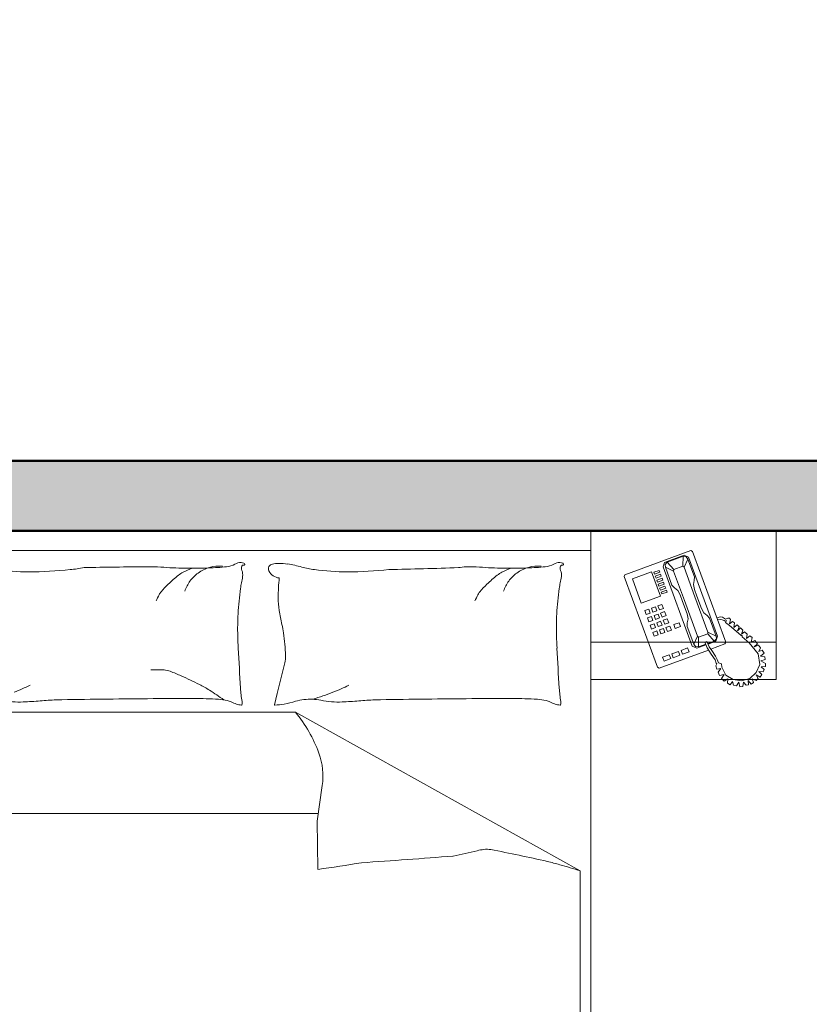
# Model space of a CAD drawing. Units: inches. Extents: x -7 to 1228, y -146 to 1091.
# Tile 32 of 88: x 680 to 747, y 446 to 531. Entities that reach past the tile are written whole.
import ezdxf

# ---------------------------------------------------------------- set-up
doc = ezdxf.new("R2010")
doc.units = ezdxf.units.IN
for name, color, linetype, lineweight in [('A-FURN', 8, 'Continuous', 18), ('A-WALL', 7, 'Continuous', 50), ('A-WALL-PATT', 251, 'Continuous', 13)]:
    doc.layers.add(name, color=color, linetype=linetype, lineweight=lineweight)
doc.styles.add('DIM_FONT', font='SIMPLEX.shx', dxfattribs={"width": 0.8})

# ---------------------------------------------------------------- blocks, each defined once
blk = doc.blocks.new('A$C4F634EDD')
for p, q in [((0.5, 2.6295), (2.3, 2.6295)), ((2.3, 2.6295), (2.3, 0.5295)), ((2.3, 2.6295), (2.8, 2.6295)), ((2.3, 2.2295), (2.3, 2.6295)), ((2.8, 2.6295), (2.8, 2.2295)), ((0.5, 2.5771), (2.3, 2.5771)), ((2.392, 2.5115), (2.5692, 2.5765)), ((2.5692, 2.5765), (2.574, 2.5743)), ((2.574, 2.5743), (2.6638, 2.3298)), ((2.4985, 2.5445), (2.5516, 2.564)), ((2.5062, 2.5454), (2.5487, 2.561)), ((2.5483, 2.5347), (2.5487, 2.561)), ((2.5487, 2.561), (2.5571, 2.56)), ((2.5615, 2.5536), (2.5514, 2.5318)), ((2.5516, 2.564), (2.5637, 2.5584)), ((2.5571, 2.56), (2.5615, 2.5536)), ((2.5615, 2.5536), (2.5791, 2.5058)), ((2.5637, 2.5584), (2.6418, 2.3458)), ((2.4842, 2.5232), (2.47, 2.518)), ((2.4862, 2.5179), (2.4842, 2.5232)), ((2.4946, 2.5331), (2.4985, 2.5445)), ((2.5734, 2.3187), (2.4946, 2.5331)), ((2.5062, 2.5454), (2.5004, 2.5392)), ((2.5004, 2.5392), (2.5013, 2.5315)), ((2.5013, 2.5315), (2.5188, 2.4836)), ((2.5013, 2.5315), (2.5231, 2.5214)), ((2.5235, 2.5256), (2.5062, 2.5454)), ((2.5231, 2.5214), (2.5235, 2.5256)), ((2.5523, 2.4417), (2.5231, 2.5214)), ((2.5483, 2.5347), (2.5235, 2.5256)), ((2.5514, 2.5318), (2.5483, 2.5347)), ((2.5807, 2.4521), (2.5514, 2.5318)), ((2.3898, 2.5066), (2.392, 2.5115)), ((2.4795, 2.2621), (2.3898, 2.5066)), ((2.412, 2.5007), (2.4634, 2.5196)), ((2.4361, 2.4352), (2.412, 2.5007)), ((2.4634, 2.5196), (2.4875, 2.454)), ((2.47, 2.518), (2.472, 2.5127)), ((2.472, 2.5127), (2.4862, 2.5179)), ((2.4881, 2.5126), (2.4739, 2.5074)), ((2.4739, 2.5074), (2.4759, 2.502)), ((2.4759, 2.502), (2.4901, 2.5073)), ((2.492, 2.5019), (2.4778, 2.4967)), ((2.4778, 2.4967), (2.4798, 2.4914)), ((2.4798, 2.4914), (2.494, 2.4966)), ((2.4901, 2.5073), (2.4881, 2.5126)), ((2.494, 2.4966), (2.492, 2.5019)), ((2.5788, 2.4956), (2.5767, 2.4848)), ((2.5791, 2.5058), (2.5788, 2.4956)), ((2.4959, 2.4913), (2.4817, 2.4861)), ((2.4817, 2.4861), (2.4837, 2.4808)), ((2.4837, 2.4808), (2.4979, 2.486)), ((2.4998, 2.4807), (2.4856, 2.4755)), ((2.4856, 2.4755), (2.4876, 2.4702)), ((2.4876, 2.4702), (2.5018, 2.4754)), ((2.5037, 2.47), (2.4895, 2.4648)), ((2.4979, 2.486), (2.4959, 2.4913)), ((2.5018, 2.4754), (2.4998, 2.4807)), ((2.5057, 2.4647), (2.5037, 2.47)), ((2.5188, 2.4836), (2.5256, 2.4761)), ((2.5256, 2.4761), (2.5342, 2.4692)), ((2.5342, 2.4692), (2.5405, 2.4574)), ((2.5767, 2.4848), (2.5795, 2.4717)), ((2.5795, 2.4717), (2.586, 2.454)), ((2.4875, 2.454), (2.4361, 2.4352)), ((2.4895, 2.4648), (2.4915, 2.4595)), ((2.4915, 2.4595), (2.5057, 2.4647)), ((2.5405, 2.4574), (2.547, 2.4397)), ((2.5523, 2.4417), (2.5875, 2.346)), ((2.5807, 2.4521), (2.6158, 2.3564)), ((2.5984, 2.4204), (2.586, 2.454)), ((2.4457, 2.4146), (2.4563, 2.4185)), ((2.4496, 2.4039), (2.4457, 2.4146)), ((2.4563, 2.4185), (2.4602, 2.4078)), ((2.4634, 2.4211), (2.474, 2.425)), ((2.4673, 2.4104), (2.4634, 2.4211)), ((2.4779, 2.4143), (2.4673, 2.4104)), ((2.474, 2.425), (2.4779, 2.4143)), ((2.4811, 2.4276), (2.4917, 2.4315)), ((2.485, 2.4169), (2.4811, 2.4276)), ((2.4956, 2.4208), (2.485, 2.4169)), ((2.4917, 2.4315), (2.4956, 2.4208)), ((2.5594, 2.4061), (2.547, 2.4397)), ((2.6047, 2.4086), (2.5984, 2.4204)), ((2.4602, 2.4078), (2.4496, 2.4039)), ((2.4528, 2.3951), (2.4635, 2.399)), ((2.4567, 2.3844), (2.4528, 2.3951)), ((2.4674, 2.3883), (2.4567, 2.3844)), ((2.4635, 2.399), (2.4674, 2.3883)), ((2.4706, 2.4016), (2.4812, 2.4055)), ((2.4745, 2.3909), (2.4706, 2.4016)), ((2.4851, 2.3949), (2.4745, 2.3909)), ((2.4812, 2.4055), (2.4851, 2.3949)), ((2.4883, 2.4081), (2.4989, 2.412)), ((2.4922, 2.3975), (2.4883, 2.4081)), ((2.5028, 2.4014), (2.4922, 2.3975)), ((2.4954, 2.3886), (2.5061, 2.3925)), ((2.4993, 2.378), (2.4954, 2.3886)), ((2.4989, 2.412), (2.5028, 2.4014)), ((2.5061, 2.3925), (2.51, 2.3819)), ((2.5622, 2.393), (2.5594, 2.4061)), ((2.5601, 2.3822), (2.5622, 2.393)), ((2.6133, 2.4017), (2.6047, 2.4086)), ((2.6201, 2.3941), (2.6133, 2.4017)), ((2.6376, 2.3463), (2.6201, 2.3941)), ((2.6499, 2.3979), (2.6397, 2.3953)), ((2.6417, 2.39), (2.6488, 2.391)), ((2.6488, 2.391), (2.6538, 2.3895)), ((2.6551, 2.397), (2.6499, 2.3979)), ((2.6538, 2.3895), (2.6596, 2.388)), ((2.6627, 2.392), (2.6551, 2.397)), ((2.6596, 2.388), (2.6626, 2.3867)), ((2.6626, 2.3867), (2.6662, 2.388)), ((2.6692, 2.394), (2.6627, 2.392)), ((2.6662, 2.388), (2.6632, 2.3828)), ((2.6736, 2.3944), (2.6692, 2.394)), ((2.6765, 2.391), (2.6736, 2.3944)), ((2.6742, 2.3795), (2.6765, 2.391)), ((2.46, 2.3756), (2.4706, 2.3795)), ((2.4639, 2.365), (2.46, 2.3756)), ((2.4745, 2.3689), (2.4639, 2.365)), ((2.4706, 2.3795), (2.4745, 2.3689)), ((2.4777, 2.3821), (2.4883, 2.386)), ((2.4816, 2.3715), (2.4777, 2.3821)), ((2.4922, 2.3754), (2.4816, 2.3715)), ((2.4849, 2.3626), (2.4955, 2.3665)), ((2.4888, 2.352), (2.4849, 2.3626)), ((2.4883, 2.386), (2.4922, 2.3754)), ((2.4955, 2.3665), (2.4994, 2.3559)), ((2.51, 2.3819), (2.4993, 2.378)), ((2.5026, 2.3691), (2.5132, 2.373)), ((2.5065, 2.3585), (2.5026, 2.3691)), ((2.5171, 2.3624), (2.5065, 2.3585)), ((2.5132, 2.373), (2.5171, 2.3624)), ((2.5238, 2.3769), (2.538, 2.3821)), ((2.5277, 2.3663), (2.5238, 2.3769)), ((2.5419, 2.3715), (2.5277, 2.3663)), ((2.538, 2.3821), (2.5419, 2.3715)), ((2.5598, 2.372), (2.5601, 2.3822)), ((2.5774, 2.3242), (2.5598, 2.372)), ((2.6632, 2.3828), (2.6736, 2.3744)), ((2.6736, 2.3744), (2.6922, 2.3593)), ((2.6824, 2.3858), (2.6742, 2.3795)), ((2.6873, 2.3815), (2.6824, 2.3858)), ((2.6853, 2.369), (2.6873, 2.3815)), ((2.6946, 2.376), (2.6853, 2.369)), ((2.6995, 2.3713), (2.6946, 2.376)), ((2.695, 2.3603), (2.6995, 2.3713)), ((2.7031, 2.3682), (2.695, 2.3603)), ((2.7096, 2.3616), (2.7031, 2.3682)), ((2.7062, 2.351), (2.7096, 2.3616)), ((2.4672, 2.3561), (2.4778, 2.36)), ((2.4711, 2.3455), (2.4672, 2.3561)), ((2.4817, 2.3494), (2.4711, 2.3455)), ((2.4778, 2.36), (2.4817, 2.3494)), ((2.4994, 2.3559), (2.4888, 2.352)), ((2.5774, 2.3242), (2.5875, 2.346)), ((2.5875, 2.346), (2.5905, 2.3431)), ((2.5905, 2.3431), (2.5901, 2.3168)), ((2.6154, 2.3522), (2.5905, 2.3431)), ((2.6158, 2.3564), (2.6154, 2.3522)), ((2.6154, 2.3522), (2.6327, 2.3324)), ((2.6376, 2.3463), (2.6158, 2.3564)), ((2.6327, 2.3324), (2.6385, 2.3386)), ((2.6418, 2.3458), (2.6369, 2.332)), ((2.6385, 2.3386), (2.6376, 2.3463)), ((2.6922, 2.3593), (2.7051, 2.3473)), ((2.7051, 2.3473), (2.7079, 2.3475)), ((2.7147, 2.3578), (2.7062, 2.351)), ((2.7079, 2.3475), (2.7079, 2.3443)), ((2.7079, 2.3443), (2.727, 2.3277)), ((2.7214, 2.3517), (2.7147, 2.3578)), ((2.7196, 2.34), (2.7214, 2.3517)), ((2.7286, 2.3466), (2.7196, 2.34)), ((2.7346, 2.3423), (2.7286, 2.3466)), ((2.732, 2.3295), (2.7346, 2.3423)), ((2.7423, 2.3345), (2.732, 2.3295)), ((2.7495, 2.325), (2.7423, 2.3345)), ((2.8, 2.3301), (2.3, 2.3301)), ((2.6172, 2.3086), (2.4844, 2.2599)), ((2.561, 2.3141), (2.5433, 2.3076)), ((2.5649, 2.3035), (2.561, 2.3141)), ((2.5855, 2.3131), (2.5734, 2.3187)), ((2.5818, 2.3178), (2.5774, 2.3242)), ((2.5901, 2.3168), (2.5818, 2.3178)), ((2.6104, 2.3222), (2.5855, 2.3131)), ((2.5901, 2.3168), (2.6097, 2.324)), ((2.613, 2.3312), (2.6077, 2.3293)), ((2.6077, 2.3293), (2.6135, 2.3141)), ((2.6192, 2.3174), (2.613, 2.3312)), ((2.6135, 2.3141), (2.6244, 2.2977)), ((2.6153, 2.3261), (2.6327, 2.3324)), ((2.6369, 2.332), (2.6161, 2.3243)), ((2.626, 2.3069), (2.6192, 2.3174)), ((2.6616, 2.3249), (2.6234, 2.3109)), ((2.6638, 2.3298), (2.6616, 2.3249)), ((2.727, 2.3277), (2.7512, 2.2983)), ((2.7406, 2.3172), (2.7495, 2.325)), ((2.7519, 2.3218), (2.7406, 2.3172)), ((2.7575, 2.3144), (2.7519, 2.3218)), ((2.7526, 2.3045), (2.7575, 2.3144)), ((2.7622, 2.308), (2.7526, 2.3045)), ((2.7673, 2.2997), (2.7622, 2.308)), ((2.5114, 2.2959), (2.4936, 2.2894)), ((2.4936, 2.2894), (2.4976, 2.2788)), ((2.4976, 2.2788), (2.5153, 2.2853)), ((2.5153, 2.2853), (2.5114, 2.2959)), ((2.5362, 2.305), (2.5185, 2.2985)), ((2.5185, 2.2985), (2.5224, 2.2879)), ((2.5224, 2.2879), (2.5401, 2.2944)), ((2.5401, 2.2944), (2.5362, 2.305)), ((2.5433, 2.3076), (2.5472, 2.297)), ((2.5472, 2.297), (2.5649, 2.3035)), ((2.6244, 2.2977), (2.6349, 2.2825)), ((2.6365, 2.2916), (2.626, 2.3069)), ((2.6349, 2.2825), (2.638, 2.273)), ((2.6407, 2.2834), (2.6365, 2.2916)), ((2.6438, 2.2739), (2.6407, 2.2834)), ((2.7512, 2.2983), (2.756, 2.2695)), ((2.7574, 2.2924), (2.7673, 2.2997)), ((2.7687, 2.2905), (2.7574, 2.2924)), ((2.7587, 2.279), (2.7699, 2.2828)), ((2.7699, 2.2828), (2.7687, 2.2905)), ((1.4546, 2.1912), (1.4752, 2.2738)), ((2.4844, 2.2599), (2.4795, 2.2621)), ((2.6399, 2.2712), (2.6374, 2.2659)), ((2.6374, 2.2659), (2.6398, 2.257)), ((2.638, 2.273), (2.6399, 2.2712)), ((2.6398, 2.257), (2.6509, 2.259)), ((2.6509, 2.259), (2.6431, 2.2492)), ((2.6519, 2.2716), (2.6438, 2.2739)), ((2.6535, 2.2628), (2.6519, 2.2716)), ((2.6636, 2.2409), (2.6535, 2.2628)), ((2.756, 2.2695), (2.7459, 2.2483)), ((2.7708, 2.2725), (2.7587, 2.279)), ((2.759, 2.2637), (2.7706, 2.2643)), ((2.7676, 2.2559), (2.759, 2.2637)), ((2.7645, 2.2498), (2.7676, 2.2559)), ((2.7706, 2.2643), (2.7708, 2.2725)), ((2.8, 2.2295), (2.3, 2.2295)), ((2.6431, 2.2492), (2.6473, 2.2398)), ((2.6473, 2.2398), (2.6592, 2.2429)), ((2.6592, 2.2429), (2.6521, 2.2314)), ((2.6521, 2.2314), (2.6598, 2.2248)), ((2.6598, 2.2248), (2.6697, 2.2309)), ((2.6836, 2.2287), (2.6636, 2.2409)), ((2.6697, 2.2309), (2.6684, 2.219)), ((2.7063, 2.2256), (2.6836, 2.2287)), ((2.7284, 2.2317), (2.7063, 2.2256)), ((2.7459, 2.2483), (2.7284, 2.2317)), ((2.7386, 2.2208), (2.7354, 2.2306)), ((2.7354, 2.2306), (2.7462, 2.2264)), ((2.7509, 2.2314), (2.7459, 2.2418)), ((2.7459, 2.2418), (2.7568, 2.2352)), ((2.7462, 2.2264), (2.7509, 2.2314)), ((2.7529, 2.2505), (2.7645, 2.2498)), ((2.7607, 2.2424), (2.7529, 2.2505)), ((2.7568, 2.2352), (2.7607, 2.2424)), ((2.6684, 2.219), (2.6761, 2.2145)), ((2.6761, 2.2145), (2.6821, 2.2237)), ((2.6821, 2.2237), (2.6843, 2.2135)), ((2.6843, 2.2135), (2.6927, 2.2117)), ((2.6927, 2.2117), (2.6986, 2.222)), ((2.6986, 2.222), (2.7019, 2.2098)), ((2.7019, 2.2098), (2.7102, 2.2104)), ((2.7102, 2.2104), (2.7113, 2.2218)), ((2.7113, 2.2218), (2.7192, 2.2137)), ((2.7192, 2.2137), (2.7255, 2.2152)), ((2.7255, 2.2152), (2.7242, 2.2265)), ((2.7242, 2.2265), (2.7324, 2.2165)), ((2.7324, 2.2165), (2.7386, 2.2208)), ((1.4471, 2.1612), (1.4546, 2.1912)), ((1.5035, 2.141), (0.5458, 2.141)), ((1.5035, 2.141), (2.2716, 1.7136)), ((1.576, 1.9433), (1.5624, 1.8479)), ((0.5458, 1.8684), (1.5653, 1.8684)), ((1.5624, 1.8479), (1.5641, 1.7178)), ((2.2716, 0.5617), (2.2716, 1.7136))]:
    blk.add_line(p, q)
for centre, radius, start, end in [((0.7851, 3.2019), 0.6827, 262.4531, 270), ((0.7851, 3.5682), 1.049, 270, 276.0867), ((0.8402, 3.0514), 0.5293, 276.0867, 280.1899), ((1.1602, -8.1346), 10.6675, 90.30153, 91.21582), ((1.1169, 2.2433), 0.2897, 85.1982, 92.5386), ((1.2142, 3.4021), 0.8732, 265.1982, 269.4243), ((1.3082, 2.3102), 0.234, 110.8603, 117.2396), ((1.2204, 4.0232), 1.4943, 269.4243, 271.9079), ((1.2995, 2.4357), 0.0992, 105.9352, 126.0864), ((1.2429, 3.3501), 0.8208, 271.9079, 275.2592), ((1.2995, 2.4357), 0.0992, 85.7841, 105.9352), ((1.3132, 2.5864), 0.0539, 275.2592, 300.6513), ((1.3554, 2.5152), 0.0289, 85.6975, 120.6513), ((1.3556, 2.519), 0.0251, 68.2117, 85.6975), ((1.3739, 2.5288), 0.0156, 158.0096, 201.421), ((1.3634, 2.533), 0.00428, 78.1069, 158.0096), ((1.3288, 2.5111), 0.0328, 351.8665, 21.421), ((1.3647, 2.5395), 0.00232, 258.1069, 19.564), ((1.3637, 2.5391), 0.00342, 19.564, 68.2117), ((1.444, 2.5274), 0.0131, 101.2724, 206.5805), ((1.4628, 2.5368), 0.0342, 206.5805, 265.5998), ((1.4591, 2.4516), 0.0904, 90, 101.2724), ((1.4591, 2.3808), 0.1611, 81.5628, 90), ((1.438, 2.2388), 0.3048, 74.256, 81.5628), ((1.5865, 2.7653), 0.2422, 254.256, 262.4531), ((1.6443, 3.2019), 0.6827, 262.4531, 270), ((1.6443, 3.5682), 1.049, 270, 276.0867), ((1.4785, 15.4878), 12.9656, 271.22425, 272.05324), ((1.97, 2.3805), 0.1524, 92.5386, 100.1899), ((1.9761, 2.2433), 0.2897, 85.1982, 92.5386), ((2.0734, 3.4021), 0.8732, 265.1982, 269.4243), ((2.1674, 2.3102), 0.234, 110.8603, 117.2396), ((2.0797, 4.0232), 1.4943, 269.4243, 271.9079), ((2.1588, 2.4357), 0.0992, 105.9352, 126.0864), ((2.1021, 3.3501), 0.8208, 271.9079, 275.2592), ((2.1588, 2.4357), 0.0992, 85.7841, 105.9352), ((2.1724, 2.5864), 0.0539, 275.2592, 300.6513), ((2.2146, 2.5152), 0.0289, 85.6975, 120.6513), ((2.2149, 2.519), 0.0251, 68.2117, 85.6975), ((2.2331, 2.5288), 0.0156, 158.0096, 201.421), ((2.2226, 2.533), 0.00428, 78.1069, 158.0096), ((2.1881, 2.5111), 0.0328, 351.8665, 21.421), ((2.224, 2.5395), 0.00232, 258.1069, 19.564), ((2.2229, 2.5391), 0.00342, 19.564, 68.2117), ((1.4317, 2.2032), 0.3916, 128.3886, 133.8115), ((1.2362, 2.45), 0.0768, 117.2396, 128.3886), ((1.2995, 2.4357), 0.0992, 143.8234, 161.5603), ((1.2995, 2.4357), 0.0992, 126.0864, 143.8234), ((1.1177, 2.5413), 0.246, 347.8905, 351.8665), ((1.949, 2.4496), 0.4918, 173.7676, 180), ((2.291, 2.2032), 0.3916, 128.3886, 133.8115), ((2.0954, 2.45), 0.0768, 117.2396, 128.3886), ((2.1588, 2.4357), 0.0992, 143.8234, 161.5603), ((2.1588, 2.4357), 0.0992, 126.0864, 143.8234), ((1.977, 2.5413), 0.246, 347.8905, 351.8665), ((1.3165, 2.3233), 0.2252, 133.8115, 140.9651), ((2.2605, 2.3525), 0.9131, 172.3191, 176.6313), ((1.5522, 2.448), 0.1983, 167.8905, 172.3191), ((2.1757, 2.3233), 0.2252, 133.8115, 140.9651), ((3.1198, 2.3525), 0.9131, 172.3191, 176.6313), ((2.4114, 2.448), 0.1983, 167.8905, 172.3191), ((1.3127, 2.3625), 0.2002, 151.6832, 156.9972), ((1.1799, 2.4341), 0.0493, 140.9651, 151.6832), ((1.6611, 2.4496), 0.204, 180, 189.6844), ((2.1719, 2.3625), 0.2002, 151.6832, 156.9972), ((2.0391, 2.4341), 0.0493, 140.9651, 151.6832), ((2.3295, 2.5637), 0.882, 189.6844, 192.1984), ((2.0266, 2.3663), 0.6787, 176.6313, 181.6331), ((2.8858, 2.3663), 0.6787, 176.6313, 181.6331), ((1.1575, 2.3103), 0.3171, 8.0051, 12.1984), ((2.7128, 2.3859), 1.3652, 181.6331, 183.055), ((0.8191, 2.2627), 0.6588, 2.6649, 8.0051), ((3.5721, 2.3859), 1.3652, 181.6331, 183.055), ((14.9657, 3.0398), 13.6356, 183.05496, 183.50486), ((15.8249, 3.0398), 13.6356, 183.05496, 183.50486), ((1.4096, 2.2902), 0.0677, 345.9548, 2.6649), ((1.1303, 1.9835), 0.2721, 85.9172, 93.5552), ((1.1455, 2.197), 0.058, 69.3257, 85.9172), ((0.9871, 1.7772), 0.5066, 65.6735, 69.3257), ((0.6058, 0.9338), 1.4323, 63.5015, 65.6735), ((0.473, 2.8815), 0.7387, 291.6577, 293.4844), ((0.473, 2.8815), 0.7387, 293.4844, 295.3111), ((1.1054, 1.9358), 0.3126, 57.865, 63.5015), ((1.6762, 2.2258), 0.3212, 183.5049, 189.9984), ((1.3322, 2.8815), 0.7387, 291.6577, 293.4844), ((1.3322, 2.8815), 0.7387, 293.4844, 295.3111), ((2.5355, 2.2258), 0.3212, 183.5049, 189.9984), ((1.2501, -19.8405), 22.0183, 90.37908, 91.01965), ((1.2012, -3.5404), 5.7185, 89.7135, 90.9704), ((1.224, 1.0141), 1.164, 86.426, 89.7135), ((0.8841, 1.5835), 0.7286, 54.1737, 57.865), ((1.2875, 2.0302), 0.1459, 77.131, 86.426), ((1.5399, 2.0561), 0.1197, 96.4341, 107.3864), ((1.5429, 2.0301), 0.1459, 78.4414, 96.4341), ((1.3322, 2.8815), 0.7387, 287.1982, 289.428), ((1.3322, 2.8815), 0.7387, 289.428, 291.6577), ((2.1093, -19.8405), 22.0183, 90.37908, 91.01965), ((2.0605, -3.5404), 5.7185, 89.7135, 90.9704), ((2.0833, 1.0141), 1.164, 86.426, 89.7135), ((2.1467, 2.0302), 0.1459, 77.131, 86.426), ((0.759, 2.3985), 0.2301, 258.4414, 272.7491), ((0.7026, 3.5718), 1.4048, 272.7491, 274.6176), ((0.9136, 0.9591), 1.2165, 92.6096, 94.6176), ((1.3099, 2.1283), 0.0453, 62.7159, 77.131), ((1.3658, 2.2367), 0.0767, 242.7159, 253.7788), ((1.3688, 2.247), 0.0875, 253.7788, 262.8796), ((1.3581, 2.1615), 0.00132, 262.8796, 343.3022), ((1.3409, 2.1667), 0.0193, 343.3022, 9.9984), ((1.448, 2.1609), 0.000917, 165.9551, 274.0829), ((1.4288, 2.4301), 0.2708, 274.0829, 279.4841), ((1.4355, 2.3896), 0.2297, 279.4841, 287.3864), ((1.6182, 2.3985), 0.2301, 258.4414, 272.7491), ((1.5619, 3.5718), 1.4048, 272.7491, 274.6176), ((1.7729, 0.9591), 1.2165, 92.6096, 94.6176), ((2.1691, 2.1283), 0.0453, 62.7159, 77.131), ((2.2251, 2.2367), 0.0767, 242.7159, 253.7788), ((2.2281, 2.247), 0.0875, 253.7788, 262.8796), ((2.2174, 2.1615), 0.00132, 262.8796, 343.3022), ((2.2001, 2.1667), 0.0193, 343.3022, 9.9984), ((1.2147, 1.9017), 0.3751, 20.1488, 39.6445), ((1.3977, 1.9688), 0.1801, 351.8644, 20.1488), ((0.6102, 18.0525), 16.3521, 273.75703, 274.62393), ((1.4194, 4.2174), 2.5158, 281.6741, 283.1904), ((2.0378, 1.5789), 0.1942, 97.7304, 103.1904), ((2.0195, 1.7137), 0.0581, 79.2724, 97.7304), ((1.2737, -2.2227), 4.0646, 77.0745, 79.2724), ((1.0582, 5.4638), 3.7801, 277.692, 279.495), ((2.0359, 1.0981), 0.6574, 74.0648, 77.0745), ((1.7125, -0.0344), 1.8351, 72.2636, 74.0648)]:
    blk.add_arc(centre, radius, start, end)
at = {"style": 'DIM_FONT', "width": 0.8, "flags": 9}
for tag, p in [('YSIZE', (0.5, 2.6295)), ('XSIZE', (0.5, 2.6295)), ('XSIZE', (2.2985, 2.6295)), ('YSIZE', (2.2985, 2.6295))]:
    blk.add_attdef(tag, p, '', height=0.0005, dxfattribs=at)

msp = doc.modelspace()

# ---------------------------------------------------------------- hatches: boundary and pattern name
at = {"layer": 'A-WALL-PATT'}
h = msp.add_hatch(color=256, dxfattribs=at)
h.dxf.hatch_style = 1
h.paths.add_polyline_path([(69, 568), (60, 568), (60, 493), (63.289, 493), (69, 493)])
h.paths.add_polyline_path([(69, 662.405), (60, 662.405), (60, 586), (69, 586)], flags=17)
h.paths.add_polyline_path([(69, 723), (184, 723), (184, 734), (179, 734), (179, 728), (69, 728), (69, 741.623), (60, 741.623), (60, 698.405), (69, 698.405)], flags=17)
h.paths.add_polyline_path([(69, 782), (231, 782), (231, 728), (231, 723), (231, 586), (236, 586), (236, 787), (69, 787), (69, 800.126), (60, 800.126), (60, 765.623), (69, 765.623)])
h.paths.add_polyline_path([(184, 842), (189, 842), (189, 848), (173, 848), (173, 842), (179, 842), (179, 787), (184, 787)])
h.paths.add_polyline_path([(118.22, 69), (69, 69), (69, 60), (118.22, 60)])
h.paths.add_polyline_path([(227, 69), (154.22, 69), (154.22, 60), (227, 60)])
h.paths.add_polyline_path([(236, 60), (232.711, 60), (227, 60), (227, 36), (236, 36)])
h.paths.add_polyline_path([(389, 60), (380, 60), (380, 36), (389, 36)])
h.paths.add_polyline_path([(384, 181), (380, 181), (380, 115), (380, 78), (384, 78)])
h.paths.add_polyline_path([(380, 115), (334.547, 115), (334.547, 109), (380, 109)])
h.paths.add_polyline_path([(274.547, 115), (236, 115), (236, 201), (232.711, 201), (231, 201), (231, 78), (236, 78), (236, 109), (274.547, 109)])
h.paths.add_polyline_path([(69, 123), (60, 123), (60, 78), (69, 78)])
h.paths.add_polyline_path([(69, 201), (60, 201), (60, 159), (69, 159)])
h.paths.add_polyline_path([(143, 219), (69, 219), (69, 213), (143, 213)], flags=17)
h.paths.add_polyline_path([(189, 219), (184, 219), (184, 274), (231, 274), (231, 219), (236, 219), (236, 279), (184, 279), (184, 297), (179, 297), (179, 279), (69, 279), (69, 290.912), (60, 290.912), (60, 262.179), (69, 262.179), (69, 274), (179, 274), (179, 219), (173, 219), (173, 213), (189, 213)])
h.paths.add_polyline_path([(69, 238.179), (60, 238.179), (60, 219), (69, 219)], flags=17)
h.paths.add_polyline_path([(69, 333), (60, 333), (60, 314.912), (69, 314.912), (69, 316.965)])
h.paths.add_polyline_path([(190, 338), (184, 338), (69, 338), (69, 333), (179, 333), (179, 327), (184, 327), (184, 333.021), (190, 333.046)])
h.paths.add_polyline_path([(69, 386.806), (60, 386.806), (60, 351), (69, 351)])
h.paths.add_polyline_path([(69, 475), (60, 475), (60, 422.806), (69, 422.806)])
h.paths.add_polyline_path([(236, 475), (231, 475), (231, 351.238), (236, 351.238)])
h.paths.add_polyline_path([(384, 475), (380, 475), (380, 362), (384, 362)])
h.paths.add_polyline_path([(547, 307), (439, 307), (439, 356), (445, 356), (445, 362), (433, 362), (433, 307), (380, 307), (380, 244), (380, 241), (384, 241), (384, 301), (433, 301), (433, 277), (439, 277), (439, 301), (547, 301)])
h.paths.add_polyline_path([(547, 241), (439, 241), (439, 247), (433, 247), (433, 235), (547, 235)])
h.paths.add_polyline_path([(450, 69), (440.286, 69), (424.889, 69), (389, 69), (389, 60), (450, 60)])
h.paths.add_polyline_path([(547, 69), (486, 69), (486, 60), (547, 60)])
h.paths.add_polyline_path([(556, 148.268), (547, 148.268), (547, 78), (556, 78)])
h.paths.add_polyline_path([(556, 223), (547, 223), (547, 195), (547, 184.268), (556, 184.268)])
h.paths.add_polyline_path([(556, 311.192), (547, 311.192), (547, 273.075), (556, 273.075)])
h.paths.add_polyline_path([(556, 344), (552.711, 344), (547, 344), (547, 335.192), (556, 335.192)])
h.paths.add_polyline_path([(556, 249.075), (547, 249.075), (547, 241), (556, 241)])
h.paths.add_polyline_path([(547, 362), (475, 362), (475, 356), (547, 356)], flags=0)
h.paths.add_polyline_path([(556, 399.621), (547, 399.621), (547, 362), (556, 362)])
h.paths.add_polyline_path([(556, 475), (547, 475), (547, 435.621), (556, 435.621)])
h.paths.add_polyline_path([(547, 493), (389, 493), (389, 487), (547, 487)])
h.paths.add_polyline_path([(380, 493), (278, 493), (278, 487), (380, 487)])
h.paths.add_polyline_path([(227, 493), (69, 493), (69, 487), (227, 487)])
h.paths.add_polyline_path([(643, 122.445), (634, 122.445), (634, 78), (643, 78)])
h.paths.add_polyline_path([(702.5, 69), (692.786, 69), (677.389, 69), (643, 69), (643, 60), (702.5, 60)])
h.paths.add_polyline_path([(798, 69), (738.5, 69), (738.5, 60), (798, 60)])
h.paths.add_polyline_path([(807, 60), (803.711, 60), (798, 60), (798, 36), (807, 36)])
h.paths.add_polyline_path([(807, 109), (846.751, 109), (846.751, 115), (807, 115), (807, 159), (802, 159), (802, 78), (807, 78)])
h.paths.add_polyline_path([(807, 201), (802, 201), (802, 195), (807, 195)])
h.paths.add_polyline_path([(643, 201), (634, 201), (634, 158.445), (643, 158.445)])
h.paths.add_polyline_path([(756, 225), (751, 225), (751, 219), (643, 219), (643, 213), (756, 213)])
h.paths.add_polyline_path([(643, 240.848), (634, 240.848), (634, 219), (643, 219)])
h.paths.add_polyline_path([(643, 274), (643, 288.629), (634, 288.629), (634, 264.848), (643, 264.848)])
h.paths.add_polyline_path([(802, 279), (756, 279), (756, 297), (751, 297), (751, 279), (643, 279), (643, 274), (751, 274), (751, 255), (756, 255), (756, 274), (802, 274)])
h.paths.add_polyline_path([(807, 333), (803.711, 333), (802, 333), (802, 279), (802, 274), (802, 219), (807, 219)])
h.paths.add_polyline_path([(956, 182), (951, 182), (951, 115), (906.751, 115), (906.751, 109), (951, 109), (951, 78), (956, 78)])
h.paths.add_polyline_path([(960, 60), (951, 60), (951, 36), (960, 36)])
h.paths.add_polyline_path([(1021, 69), (1005.781, 69), (960, 69), (960, 60), (1021, 60)])
h.paths.add_polyline_path([(956, 224), (951, 224), (951, 218), (956, 218)])
h.paths.add_polyline_path([(956, 302), (1004, 302), (1004, 278), (1010, 278), (1010, 302), (1118, 302), (1118, 290.809), (1127, 290.809), (1127, 326.968), (1118, 326.968), (1118, 320.966), (1118, 307), (1010, 307), (1010, 356), (1016, 356), (1016, 362), (1004, 362), (1004, 307), (951, 307), (951, 244), (951, 242), (954.289, 242), (956, 242)])
h.paths.add_polyline_path([(643, 333), (634, 333), (634, 312.629), (643, 312.629), (643, 316.965)])
h.paths.add_polyline_path([(756, 338), (643, 338), (643, 333), (751, 333), (751, 327), (756, 327)])
h.paths.add_polyline_path([(643, 388), (634, 388), (634, 351), (643, 351)])
h.paths.add_polyline_path([(807, 357), (802, 357), (802, 351), (807, 351)])
h.paths.add_polyline_path([(807, 475), (802, 475), (802, 393), (807, 393)])
h.paths.add_polyline_path([(643, 475), (634, 475), (634, 424), (643, 424)])
h.paths.add_polyline_path([(798, 493), (643, 493), (643, 487), (798, 487)])
h.paths.add_polyline_path([(634, 493), (556, 493), (556, 487), (634, 487)])
h.paths.add_polyline_path([(813, 493), (807, 493), (807, 487), (813, 487)])
h.paths.add_polyline_path([(951, 493), (849, 493), (849, 487), (951, 487)])
h.paths.add_polyline_path([(956, 484), (951, 484), (951, 374), (956, 374)])
h.paths.add_polyline_path([(1109, 493), (969, 493), (969, 487), (1109, 487)])
h.paths.add_polyline_path([(1127, 484), (1118, 484), (1118, 450.641), (1127, 450.641)])
h.paths.add_polyline_path([(1127, 414.641), (1118, 414.641), (1118, 365), (1127, 365)])
h.paths.add_polyline_path([(1109, 362), (1046, 362), (1046, 356), (1109, 356)], flags=17)
h.paths.add_polyline_path([(1127, 356), (1123.454, 356), (1118, 356), (1118, 350.968), (1127, 350.968)], flags=0)
h.paths.add_polyline_path([(1127, 266.809), (1118, 266.809), (1118, 262.361), (1118, 242), (1127, 242)], flags=17)
h.paths.add_polyline_path([(1118, 242), (1010, 242), (1010, 248), (1004, 248), (1004, 237), (1118, 237)])
h.paths.add_polyline_path([(1127, 224), (1118, 224), (1118, 170), (1127, 170)])
h.paths.add_polyline_path([(1127, 134), (1118, 134), (1118, 78), (1127, 78)])
h.paths.add_polyline_path([(1118, 69), (1057, 69), (1057, 60), (1118, 60)])
h.paths.add_polyline_path([(227, 571.546), (227, 574), (69, 574), (69, 568), (227, 568)])
h.paths.add_polyline_path([(380, 571.546), (380, 574), (278, 574), (278, 568), (380, 568)])
h.paths.add_polyline_path([(242, 574), (236, 574), (236, 568), (242, 568)])
h.paths.add_polyline_path([(547, 571.546), (547, 574), (389, 574), (389, 568), (547, 568)])
h.paths.add_polyline_path([(384, 733), (380, 733), (380, 586), (384, 586)])
h.paths.add_polyline_path([(556, 646), (634, 646), (634, 655), (547, 655), (547, 586), (556, 586)])
h.paths.add_polyline_path([(634, 574), (556, 574), (556, 568), (634, 568)])
h.paths.add_polyline_path([(643, 655), (634, 655), (634, 586), (643, 586)])
h.paths.add_polyline_path([(798, 574), (643, 574), (643, 568), (798, 568)])
h.paths.add_polyline_path([(643, 663.854), (634, 663.854), (634, 655), (643, 655)])
h.paths.add_polyline_path([(556, 676.967), (547, 676.967), (547, 655), (556, 655)])
h.paths.add_polyline_path([(556, 733), (547, 733), (547, 712.967), (556, 712.967)])
h.paths.add_polyline_path([(643, 710), (634, 710), (634, 699.854), (643, 699.854)])
h.paths.add_polyline_path([(807, 668), (802, 668), (802, 586), (807, 586)])
h.paths.add_polyline_path([(951, 574), (849, 574), (849, 568), (951, 568)])
h.paths.add_polyline_path([(956, 691), (951, 691), (951, 577), (956, 577)])
h.paths.add_polyline_path([(1109, 574), (969, 574), (969, 568), (1109, 568)])
h.paths.add_polyline_path([(1127, 643.403), (1118, 643.403), (1118, 577), (1127, 577)])
h.paths.add_polyline_path([(1127, 568), (1123.454, 568), (1118, 568), (1118, 493), (1127, 493)])
h.paths.add_polyline_path([(1127, 733), (1118, 733), (1118, 679.403), (1127, 679.403)])
h.paths.add_polyline_path([(1127, 777.348), (1118, 777.348), (1118, 770.035), (1118, 751), (1127, 751)], flags=17)
h.paths.add_polyline_path([(1118, 751), (1010, 751), (1010, 757), (1004, 757), (1004, 745), (1118, 745)])
h.paths.add_polyline_path([(956, 811), (1004, 811), (1004, 787), (1010, 787), (1010, 811), (1017.874, 811), (1017.874, 811.627, -0.414214), (1018.247, 812), (1031.978, 812, -0.414214), (1032.351, 811.627), (1032.351, 811), (1118, 811), (1118, 801.348), (1127, 801.348), (1127, 834.685), (1118, 834.685), (1118, 830.238), (1118, 817), (1010, 817), (1010, 866), (1016, 866), (1016, 872), (1004, 872), (1004, 817), (956, 817), (956, 866), (951, 866), (951, 751), (954.289, 751), (956, 751)])
h.paths.add_polyline_path([(1118, 872), (1046, 872), (1046, 866), (1118, 866)], flags=17)
h.paths.add_polyline_path([(1127, 924.711), (1118, 924.711), (1118, 884), (1127, 884)])
h.paths.add_polyline_path([(1127, 866), (1123.711, 866), (1118, 866), (1118, 858.685), (1127, 858.685)], flags=17)
h.paths.add_polyline_path([(956, 983), (951, 983), (951, 952), (807, 952), (807, 983), (802, 983), (802, 902), (807, 902), (807, 946), (951, 946), (951, 884), (956, 884)])
h.paths.add_polyline_path([(807, 842), (802, 842), (802, 787), (756, 787), (756, 806), (751, 806), (751, 787), (643, 787), (643, 782), (751, 782), (751, 764), (756, 764), (756, 782), (802, 782), (802, 728), (807, 728)])
h.paths.add_polyline_path([(756, 848), (643, 848), (643, 842), (751, 842), (751, 836), (756, 836)])
h.paths.add_polyline_path([(756, 734), (751, 734), (751, 728), (643, 728), (643, 723), (756, 723)])
h.paths.add_polyline_path([(643, 749.791), (634, 749.791), (634, 728), (637.289, 728), (643, 728)])
h.paths.add_polyline_path([(643, 805.405), (634, 805.405), (634, 773.791), (643, 773.791)])
h.paths.add_polyline_path([(643, 896.663), (634, 896.663), (634, 860), (637.289, 860), (643, 860)])
h.paths.add_polyline_path([(643, 842), (634, 842), (634, 829.405), (643, 829.405)])
h.paths.add_polyline_path([(643, 983), (634, 983), (634, 932.663), (643, 932.663)])
h.paths.add_polyline_path([(1127, 983), (1118, 983), (1118, 960.711), (1127, 960.711)])
h.paths.add_polyline_path([(1118, 1001), (1077.525, 1001), (1077.525, 992), (1118, 992)])
h.paths.add_polyline_path([(1041.525, 1001), (960, 1001), (960, 992), (1041.525, 992)])
h.paths.add_polyline_path([(960, 1025), (951, 1025), (951, 1001), (954.289, 1001), (960, 1001)])
h.paths.add_polyline_path([(807, 1025), (798, 1025), (798, 1001), (807, 1001)])
h.paths.add_polyline_path([(798, 1001), (738.5, 1001), (738.5, 992), (798, 992)])
h.paths.add_polyline_path([(702.5, 1001), (643, 1001), (643, 992), (702.5, 992)])
h.paths.add_polyline_path([(547, 1001), (499.113, 1001), (499.113, 992), (547, 992)])
h.paths.add_polyline_path([(463.113, 1001), (389, 1001), (389, 992), (463.113, 992)])
h.paths.add_polyline_path([(389, 1025), (380, 1025), (380, 1022), (380, 1001), (383.289, 1001), (389, 1001)])
h.paths.add_polyline_path([(236, 1025), (227, 1025), (227, 1001), (236, 1001)])
h.paths.add_polyline_path([(236, 983), (231, 983), (231, 860), (236, 860)])
h.paths.add_polyline_path([(274.547, 952), (236, 952), (236, 946), (274.547, 946)])
h.paths.add_polyline_path([(380, 952), (334.547, 952), (334.547, 946), (380, 946)])
h.paths.add_polyline_path([(384, 983), (380, 983), (380, 884), (383.289, 884), (384, 884)])
h.paths.add_polyline_path([(227, 1001), (155.012, 1001), (155.012, 992), (162.875, 992), (227, 992)])
h.paths.add_polyline_path([(119.012, 1001), (69, 1001), (69, 992), (119.012, 992)])
h.paths.add_polyline_path([(69, 983), (60, 983), (60, 922.987), (69, 922.987)])
h.paths.add_polyline_path([(69, 886.987), (60, 886.987), (60, 860), (63.289, 860), (69, 860)])
h.paths.add_polyline_path([(143, 848), (69, 848), (69, 842), (143, 842)])

# ---------------------------------------------------------------- linework, layer by layer
at = {"layer": 'A-WALL'}
for p, q in [((813, 493), (556, 493)), ((813, 487), (556, 487))]:
    msp.add_line(p, q, dxfattribs=at)

# ---------------------------------------------------------------- block references
at = {"layer": 'A-FURN', "xscale": 31.78426361944092, "yscale": 31.78426361944092, "zscale": 31.78426361944092}
msp.add_blockref('A$C4F634EDD', (655.397, 403.423), dxfattribs=at)

doc.saveas('drawing.dxf')
